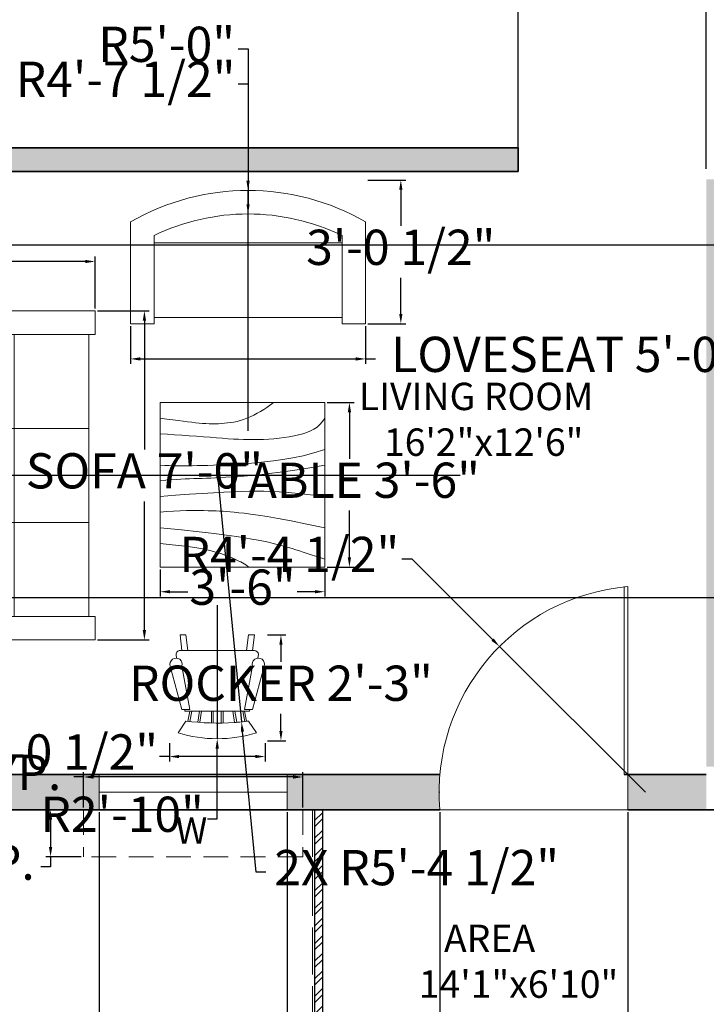
# Model space of a CAD drawing. Units: inches. Extents: x 9689 to 10369, y 10965 to 11626.
# Tile 3 of 11: x 9830 to 10005, y 11108 to 11359. Entities that reach past the tile are written whole.
import ezdxf

# ---------------------------------------------------------------- set-up
doc = ezdxf.new("R2010")
doc.units = ezdxf.units.IN
doc.linetypes.add('ACAD_ISO02W100', pattern=[15, 12, -3])
doc.linetypes.add('DASHED2', pattern=[9.525, 6.35, -3.175])
for name, color, linetype, lineweight in [('A-ANNO-DIMS', 2, 'Continuous', 18), ('A-ANNO-TEXT', 7, 'Continuous', 18), ('A-AREA-IDEN', 7, 'Continuous', 18), ('A-DOOR', 4, 'Continuous', 18), ('A-FLOR', 7, 'Continuous', 25), ('A-FLOR-PATT', 252, 'Continuous', 13), ('A-FURN', 8, 'Continuous', 18), ('A-GLAZ', 4, 'Continuous', 18), ('A-GLAZ-OVHD', 4, 'DASHED2', 13), ('A-WALL', 7, 'Continuous', 35), ('A-WALL-PATT', 252, 'Continuous', 13), ('C-PARK', 7, 'ACAD_ISO02W100', 18)]:
    doc.layers.add(name, color=color, linetype=linetype, lineweight=lineweight)
doc.styles.get("Standard").update_dxf_attribs({"font": 'arial.ttf'})
doc.dimstyles.new('ISO-25', dxfattribs={"dimtxt": 9, "dimasz": 2.5, "dimexe": 1.25, "dimexo": 0.625, "dimgap": 2, "dimtad": 0, "dimtih": 1, "dimtoh": 1, "dimdec": 1, "dimlunit": 4, "dimtxsty": 'Standard', "dimcen": 2.5, "dimadec": 0, "dimazin": 0, "dimtfac": 0.5, "dimtdec": 1, "dimtmove": 0, "dimatfit": 3, "dimfxl": 1, "dimarcsym": 0})

# ---------------------------------------------------------------- blocks, each defined once
blk = doc.blocks.new('Sofa - Roundback 7 ft.')
for p, q in [((-12.00002, -32.4421), (-12.00003, -6.5971)), ((11.99997, -32.4421), (11.99998, -6.5971)), ((-36.000027, -34), (-36.000027, -11.4696)), ((35.99998, -34), (35.99998, -11.4696)), ((-35.999844, -13.3819), (35.9998, -13.3819)), ((-36.000027, -32.4421), (35.99998, -32.4421))]:
    blk.add_line(p, q)
for points in [[(-36.000027, -34), (-42.000027, -34), (-42.000027, -8)], [(41.99998, -8), (41.99998, -34), (35.99998, -34)]]:
    blk.add_lwpolyline(points)
for centre, radius, start, end in [((0, -114.25), 114.25, 68.43141, 111.5686), ((-0.00001, -127.1968), 121.1968, 72.72033, 107.2797)]:
    blk.add_arc(centre, radius, start, end)
blk = doc.blocks.new('Sofa - Roundback Loveseat 5 ft.')
for p, q in [((0, -32.44198), (0, -5.99998)), ((-24, -33.99998), (-24, -11.46958)), ((24.00004, -33.99998), (24.00004, -11.46958)), ((-23.9998, -13.38178), (23.99986, -13.38178)), ((-24, -32.44198), (24.00004, -32.44198))]:
    blk.add_line(p, q)
for points in [[(-24, -33.99998), (-30, -33.99998), (-30, -7.99998)], [(30.00004, -7.99998), (30.00004, -33.99998), (24.00004, -33.99998)]]:
    blk.add_lwpolyline(points)
for centre, radius, start, end in [((0, -60.24998), 60.24998, 60.13715, 119.8628), ((0, -61.38438), 55.38444, 64.32083, 115.6792)]:
    blk.add_arc(centre, radius, start, end)
blk = doc.blocks.new('Chair - Rocking')
for p, q in [((-8, -4.5), (-10, -1.5)), ((8, -4.5), (10, -1.5)), ((-7.5, -4.5), (-7, -7)), ((-6.5, -7), (-7.02225, -4.43)), ((-4.5, -7), (-4.96674, -4.19951)), ((-4, -7), (-4.40532, -4.16272)), ((-1.5, -4.05012), (-1.5, -7)), ((-1, -7), (-1, -4.05012)), ((1, -7), (1, -4.04655)), ((1.5, -4.05012), (1.5, -7)), ((4, -7), (4.40187, -4.18694)), ((4.5, -7), (4.96761, -4.19437)), ((6.5, -7), (7, -4.4057)), ((7.5, -4.5), (7, -7)), ((-9, -7.5), (-12, -18.49999)), ((-7, -7.5), (-9, -7.5)), ((-9, -18.49999), (-7, -7.5)), ((-8.23428, -6.99939), (-8.3093, -7.47958)), ((-8.23041, -7), (8.23915, -7)), ((7, -7.5), (9, -7.5)), ((9, -18.49999), (7, -7.5)), ((8.31071, -7.48854), (8.23449, -7.00073)), ((9, -7.5), (12, -18.49999)), ((-10.36644, -20.64523), (-10.5, -21.49999)), ((-9, -22.49999), (-9.5, -26.49999)), ((0, -22.49999), (-9.5, -22.49999)), ((-8, -26.49999), (-7.5, -22.49999)), ((0, -22.49999), (9.5, -22.49999)), ((8, -26.49999), (7.5, -22.49999)), ((9, -22.49999), (9.5, -26.49999)), ((10.5, -21.49999), (10.3575, -20.58798)), ((-9.5, -26.49999), (-8, -26.49999)), ((9.5, -26.49999), (8, -26.49999))]:
    blk.add_line(p, q)
for centre, radius, start, end in [((0, -34.08333), 34.08333, 72.93847, 107.0615), ((0, -68.25004), 64.25, 93.92211, 97.15267), ((0, -68.25004), 64.25, 82.84733, 93.92211), ((-10.5, -18.99999), 1.58114, 161.5651, 18.43495), ((10.5, -18.99999), 1.58114, 161.5651, 18.43495), ((-9.5, -21.49999), 1, 180, 270), ((9.5, -21.49999), 1, 270, 0)]:
    blk.add_arc(centre, radius, start, end)
blk = doc.blocks.new('Table - Square Woodgrain 42 x 42 in.')
blk.add_line((0, -42), (42, -42))
for points in [[(0, -4), (1.704, -4.2172), (3.2358, -4.4188), (4.615, -4.604), (5.8615, -4.7721), (6.9951, -4.9224), (8.0357, -5.0541), (9.0031, -5.1667), (9.9171, -5.2594), (10.7951, -5.3316), (11.6445, -5.3836), (12.4702, -5.4157), (13.277, -5.4283), (14.0698, -5.4217), (14.8535, -5.3964), (15.6331, -5.3526), (16.4133, -5.2908), (17.1986, -5.2103), (17.9913, -5.1062), (18.793, -4.9727), (19.6056, -4.8038), (20.4307, -4.5937), (21.2701, -4.3365), (22.1256, -4.0262), (22.9989, -3.6571), (23.888, -3.2272), (24.7756, -2.7516), (25.6408, -2.2491), (26.4624, -1.7387), (27.2195, -1.2395), (27.891, -0.7703), (28.456, -0.3501), (28.8934, 0.002)], [(0, -42), (0, 0), (42, 0), (42, -42)], [(0, -8), (1.8203, -8.1001), (3.6741, -8.2149), (5.5411, -8.3408), (7.4011, -8.4741), (9.2339, -8.6112), (11.0193, -8.7484), (12.7371, -8.8821), (14.3671, -9.0086), (15.8954, -9.1246), (17.3337, -9.2278), (18.6997, -9.3159), (20.0116, -9.387), (21.2871, -9.4389), (22.5442, -9.4696), (23.8008, -9.477), (25.0749, -9.459), (26.3791, -9.4137), (27.7049, -9.3403), (29.0383, -9.2382), (30.3655, -9.1068), (31.6728, -8.9455), (32.9461, -8.7535), (34.1717, -8.5304), (35.3358, -8.2756), (36.4268, -7.9863), (37.443, -7.6521), (38.3849, -7.2603), (39.253, -6.7986), (40.048, -6.2542), (40.7705, -5.6147), (41.421, -4.8674), (42, -4)], [(42, -12), (39.1784, -12.8621), (36.4519, -13.5654), (33.8246, -14.1294), (31.3004, -14.5731), (28.8832, -14.9161), (26.577, -15.1775), (24.3858, -15.3768), (22.3136, -15.5332), (20.3622, -15.6632), (18.5254, -15.7718), (16.7947, -15.8612), (15.1618, -15.9338), (13.6183, -15.9916), (12.1558, -16.0369), (10.7659, -16.0718), (9.4403, -16.0987), (8.1703, -16.1191), (6.9461, -16.1325), (5.7577, -16.1377), (4.595, -16.1335), (3.4479, -16.1188), (2.3064, -16.0924), (1.1604, -16.0532), (0, -16)], [(42, -16), (37.6529, -16.7365), (33.8802, -17.329), (30.6179, -17.7961), (27.8015, -18.1561), (25.3668, -18.4275), (23.2497, -18.6288), (21.3859, -18.7785), (19.7111, -18.8949), (18.1693, -18.9939), (16.7375, -19.0795), (15.401, -19.1534), (14.1449, -19.217), (12.9544, -19.2717), (11.8148, -19.3191), (10.7113, -19.3606), (9.6291, -19.3976), (8.5534, -19.4323), (7.47, -19.4689), (6.3643, -19.5122), (5.222, -19.5672), (4.0288, -19.6386), (2.7703, -19.7313), (1.4321, -19.8501), (0, -20)], [(0, -24), (3.9243, -23.6805), (7.4766, -23.4138), (10.6891, -23.1954), (13.5943, -23.0205), (16.2247, -22.8847), (18.6125, -22.7832), (20.7903, -22.7116), (22.7903, -22.6651), (24.6563, -22.642), (26.4764, -22.6507), (28.35, -22.7024), (30.3766, -22.8084), (32.6555, -22.98), (35.2861, -23.2283), (38.3678, -23.5645), (42, -24)], [(42, -32), (37.392, -31.017), (33.4585, -30.2231), (30.1291, -29.5949), (27.3334, -29.109), (25.0009, -28.742), (23.0612, -28.4707), (21.4439, -28.2716), (20.0786, -28.1215), (18.8998, -28.0002), (17.8609, -27.9014), (16.9206, -27.8219), (16.0371, -27.7588), (15.1691, -27.709), (14.2748, -27.6693), (13.3128, -27.6368), (12.2415, -27.6083), (11.0295, -27.5824), (9.6867, -27.5643), (8.233, -27.5608), (6.6884, -27.5787), (5.0728, -27.6248), (3.4062, -27.7058), (1.7086, -27.8286), (0, -28)], [(0, -32), (5.4026, -32.5358), (9.9494, -33.019), (13.7424, -33.4553), (16.8834, -33.8505), (19.4743, -34.2106), (21.6171, -34.5413), (23.4136, -34.8486), (24.9657, -35.1382), (26.3614, -35.4156), (27.6332, -35.6841), (28.7995, -35.9467), (29.8788, -36.2064), (30.8897, -36.4661), (31.8507, -36.7288), (32.7802, -36.9973), (33.6968, -37.2747), (34.6175, -37.5635), (35.5531, -37.8651), (36.5128, -38.1805), (37.506, -38.5108), (38.5421, -38.8568), (39.6302, -39.2197), (40.7797, -39.6004), (42, -40)], [(0, -36), (3.0098, -36.2857), (5.5354, -36.5643), (7.6368, -36.8359), (9.374, -37.1009), (10.807, -37.3597), (11.9957, -37.6126), (13.0002, -37.8599), (13.8804, -38.102), (14.6874, -38.3393), (15.4365, -38.5729), (16.1338, -38.8041), (16.7858, -39.0341), (17.3987, -39.264), (17.9787, -39.4952), (18.5322, -39.7288), (19.0655, -39.9662), (19.5832, -40.2081), (20.0842, -40.4544), (20.5657, -40.7046), (21.0249, -40.9581), (21.459, -41.2144), (21.8653, -41.4731), (22.2409, -41.7335), (22.5831, -41.9951)]]:
    blk.add_lwpolyline(points)
blk = doc.blocks.new('WINDOW-HOOD-56')
for p, q in [((0, 0), (0, 12)), ((0, 12), (56, 12)), ((56, 0), (56, 12))]:
    blk.add_line(p, q)
blk = doc.blocks.new('WINDOW-48')
for p, q in [((0, 0), (0, 9)), ((48, 0), (48, 9)), ((0, 4.5), (48, 4.5))]:
    blk.add_line(p, q)
blk = doc.blocks.new('*D38')
at = {"layer": 'A-ANNO-DIMS', "color": 0, "lineweight": -2, "transparency": 16777216}
for p, q in [((9846.06, 11166.03), (9843.56, 11166.03)), ((9846.06, 11158.26), (9846.06, 11167.28)), ((9899.56, 11166.03), (9848.56, 11166.03)), ((9902.06, 11158.26), (9902.06, 11167.28))]:
    blk.add_line(p, q, dxfattribs=at)
at = {"layer": 'A-ANNO-DIMS', "color": 0, "transparency": 16777216}
for points in [[(9848.56, 11166.45), (9848.56, 11165.61), (9846.06, 11166.03)], [(9899.56, 11166.45), (9899.56, 11165.61), (9902.06, 11166.03)]]:
    blk.add_solid(points, dxfattribs=at)
at = {"layer": 'Defpoints', "color": 0, "transparency": 16777216}
for p in [(9846.06, 11166.03), (9846.06, 11157.63), (9902.06, 11157.63)]:
    blk.add_point(p, dxfattribs=at)
at = {"layer": 'A-ANNO-DIMS', "color": 0, "transparency": 16777216, "insert": (9793.76, 11166.03), "char_height": 9, "attachment_point": 5}
blk.add_mtext('HOOD 4\'-8" TYP.', dxfattribs=at)
blk = doc.blocks.new('*D39')
at = {"layer": 'A-ANNO-DIMS', "color": 0, "lineweight": -2, "transparency": 16777216}
for p, q in [((9845.43, 11157.63), (9836.41, 11157.63)), ((9837.66, 11155.13), (9837.66, 11148.13)), ((9845.43, 11145.63), (9836.41, 11145.63)), ((9837.66, 11145.63), (9837.66, 11143.13)), ((9837.66, 11143.13), (9835.16, 11143.13))]:
    blk.add_line(p, q, dxfattribs=at)
at = {"layer": 'A-ANNO-DIMS', "color": 0, "transparency": 16777216}
for points in [[(9837.24, 11155.13), (9838.07, 11155.13), (9837.66, 11157.63)], [(9837.24, 11148.13), (9838.07, 11148.13), (9837.66, 11145.63)]]:
    blk.add_solid(points, dxfattribs=at)
at = {"layer": 'Defpoints', "color": 0, "transparency": 16777216}
for p in [(9846.06, 11157.63), (9837.66, 11145.63), (9846.06, 11145.63)]:
    blk.add_point(p, dxfattribs=at)
at = {"layer": 'A-ANNO-DIMS', "color": 0, "transparency": 16777216, "insert": (9806.15, 11143.13), "char_height": 9, "attachment_point": 5}
blk.add_mtext('1\'-0" TYP.', dxfattribs=at)
blk = doc.blocks.new('*D54')
at = {"layer": 'A-ANNO-DIMS', "color": 0, "lineweight": -2, "transparency": 16777216}
for p, q in [((9849.64, 11285.02), (9862.86, 11285.02)), ((9861.61, 11282.52), (9861.61, 11249.67)), ((9861.61, 11203.52), (9861.61, 11236.36)), ((9849.64, 11201.02), (9862.86, 11201.02))]:
    blk.add_line(p, q, dxfattribs=at)
at = {"layer": 'A-ANNO-DIMS', "color": 0, "transparency": 16777216}
for points in [[(9861.19, 11282.52), (9862.03, 11282.52), (9861.61, 11285.02)], [(9861.19, 11203.52), (9862.03, 11203.52), (9861.61, 11201.02)]]:
    blk.add_solid(points, dxfattribs=at)
at = {"layer": 'Defpoints', "color": 0, "transparency": 16777216}
for p in [(9849.01, 11285.02), (9861.61, 11285.02), (9849.01, 11201.02)]:
    blk.add_point(p, dxfattribs=at)
at = {"layer": 'A-ANNO-DIMS', "color": 0, "transparency": 16777216, "insert": (9861.61, 11243.02), "char_height": 9, "attachment_point": 5}
blk.add_mtext('SOFA 7\'-0"', dxfattribs=at)
blk = doc.blocks.new('*D55')
at = {"layer": 'A-ANNO-DIMS', "color": 0, "lineweight": -2, "transparency": 16777216}
for p, q in [((9812.34, 11285.64), (9812.34, 11298.87)), ((9849.01, 11285.64), (9849.01, 11298.87)), ((9812.34, 11297.62), (9809.84, 11297.62)), ((9846.51, 11297.62), (9814.84, 11297.62))]:
    blk.add_line(p, q, dxfattribs=at)
at = {"layer": 'A-ANNO-DIMS', "color": 0, "transparency": 16777216}
for points in [[(9814.84, 11298.03), (9814.84, 11297.2), (9812.34, 11297.62)], [(9846.51, 11298.03), (9846.51, 11297.2), (9849.01, 11297.62)]]:
    blk.add_solid(points, dxfattribs=at)
at = {"layer": 'Defpoints', "color": 0, "transparency": 16777216}
for p in [(9812.34, 11297.62), (9812.34, 11285.02), (9849.01, 11285.02)]:
    blk.add_point(p, dxfattribs=at)
at = {"layer": 'A-ANNO-DIMS', "color": 0, "transparency": 16777216, "insert": (9785.4, 11297.62), "char_height": 9, "attachment_point": 5}
blk.add_mtext('3\'-0 1/2"', dxfattribs=at)
blk = doc.blocks.new('*D56')
at = {"layer": 'A-ANNO-DIMS', "color": 0, "lineweight": -2, "transparency": 16777216}
for p, q in [((9858.07, 11281.13), (9858.07, 11271.5)), ((9918.07, 11281.13), (9918.07, 11271.5)), ((9860.57, 11272.75), (9915.57, 11272.75)), ((9918.07, 11272.75), (9920.57, 11272.75))]:
    blk.add_line(p, q, dxfattribs=at)
at = {"layer": 'A-ANNO-DIMS', "color": 0, "transparency": 16777216}
for points in [[(9860.57, 11273.17), (9860.57, 11272.33), (9858.07, 11272.75)], [(9915.57, 11273.17), (9915.57, 11272.33), (9918.07, 11272.75)]]:
    blk.add_solid(points, dxfattribs=at)
at = {"layer": 'Defpoints', "color": 0, "transparency": 16777216}
for p in [(9858.07, 11281.75), (9918.07, 11281.75), (9918.07, 11272.75)]:
    blk.add_point(p, dxfattribs=at)
at = {"layer": 'A-ANNO-DIMS', "color": 0, "transparency": 16777216, "insert": (9969.27, 11272.75), "char_height": 9, "attachment_point": 5}
blk.add_mtext('LOVESEAT 5\'-0"', dxfattribs=at)
blk = doc.blocks.new('*D57')
at = {"layer": 'A-ANNO-DIMS', "color": 0, "lineweight": -2, "transparency": 16777216}
for p, q in [((9918.69, 11318.42), (9928.32, 11318.42)), ((9927.07, 11315.92), (9927.07, 11306.74)), ((9927.07, 11284.25), (9927.07, 11293.43)), ((9918.69, 11281.75), (9928.32, 11281.75))]:
    blk.add_line(p, q, dxfattribs=at)
at = {"layer": 'A-ANNO-DIMS', "color": 0, "transparency": 16777216}
for points in [[(9926.65, 11315.92), (9927.49, 11315.92), (9927.07, 11318.42)], [(9926.65, 11284.25), (9927.49, 11284.25), (9927.07, 11281.75)]]:
    blk.add_solid(points, dxfattribs=at)
at = {"layer": 'Defpoints', "color": 0, "transparency": 16777216}
for p in [(9918.07, 11318.42), (9927.07, 11318.42), (9918.07, 11281.75)]:
    blk.add_point(p, dxfattribs=at)
at = {"layer": 'A-ANNO-DIMS', "color": 0, "transparency": 16777216, "insert": (9927.07, 11300.08), "char_height": 9, "attachment_point": 5}
blk.add_mtext('3\'-0 1/2"', dxfattribs=at)
blk = doc.blocks.new('*D58')
at = {"layer": 'A-ANNO-DIMS', "color": 0, "lineweight": -2, "transparency": 16777216}
for p, q in [((9893.04, 11202.3), (9897.72, 11202.3)), ((9896.47, 11199.8), (9896.47, 11195.46)), ((9896.47, 11177.8), (9896.47, 11182.14)), ((9893.04, 11175.3), (9897.72, 11175.3))]:
    blk.add_line(p, q, dxfattribs=at)
at = {"layer": 'A-ANNO-DIMS', "color": 0, "transparency": 16777216}
for points in [[(9896.05, 11199.8), (9896.88, 11199.8), (9896.47, 11202.3)], [(9896.05, 11177.8), (9896.88, 11177.8), (9896.47, 11175.3)]]:
    blk.add_solid(points, dxfattribs=at)
at = {"layer": 'Defpoints', "color": 0, "transparency": 16777216}
for p in [(9892.42, 11202.3), (9892.42, 11175.3), (9896.47, 11175.3)]:
    blk.add_point(p, dxfattribs=at)
at = {"layer": 'A-ANNO-DIMS', "color": 0, "transparency": 16777216, "insert": (9896.47, 11188.8), "char_height": 9, "attachment_point": 5}
blk.add_mtext('ROCKER 2\'-3"', dxfattribs=at)
blk = doc.blocks.new('*D59')
at = {"layer": 'A-ANNO-DIMS', "color": 0, "lineweight": -2, "transparency": 16777216}
for p, q in [((9867.98, 11174.67), (9867.98, 11170)), ((9892.42, 11174.67), (9892.42, 11170)), ((9867.98, 11171.25), (9865.48, 11171.25)), ((9889.92, 11171.25), (9870.48, 11171.25))]:
    blk.add_line(p, q, dxfattribs=at)
at = {"layer": 'A-ANNO-DIMS', "color": 0, "transparency": 16777216}
for points in [[(9870.48, 11171.67), (9870.48, 11170.83), (9867.98, 11171.25)], [(9889.92, 11171.67), (9889.92, 11170.83), (9892.42, 11171.25)]]:
    blk.add_solid(points, dxfattribs=at)
at = {"layer": 'Defpoints', "color": 0, "transparency": 16777216}
for p in [(9867.98, 11175.3), (9892.42, 11175.3), (9867.98, 11171.25)]:
    blk.add_point(p, dxfattribs=at)
at = {"layer": 'A-ANNO-DIMS', "color": 0, "transparency": 16777216, "insert": (9840.96, 11171.25), "char_height": 9, "attachment_point": 5}
blk.add_mtext('2\'-0 1/2"', dxfattribs=at)
blk = doc.blocks.new('*D60')
at = {"layer": 'A-ANNO-DIMS', "color": 0, "lineweight": -2, "transparency": 16777216}
for p, q in [((9908.27, 11261.62), (9915.2, 11261.62)), ((9913.95, 11259.12), (9913.95, 11247.22)), ((9913.95, 11222.12), (9913.95, 11234.03)), ((9908.27, 11219.62), (9915.2, 11219.62))]:
    blk.add_line(p, q, dxfattribs=at)
at = {"layer": 'A-ANNO-DIMS', "color": 0, "transparency": 16777216}
for points in [[(9913.53, 11259.12), (9914.37, 11259.12), (9913.95, 11261.62)], [(9913.53, 11222.12), (9914.37, 11222.12), (9913.95, 11219.62)]]:
    blk.add_solid(points, dxfattribs=at)
at = {"layer": 'Defpoints', "color": 0, "transparency": 16777216}
for p in [(9907.65, 11261.62), (9913.95, 11261.62), (9907.65, 11219.62)]:
    blk.add_point(p, dxfattribs=at)
at = {"layer": 'A-ANNO-DIMS', "color": 0, "transparency": 16777216, "insert": (9913.95, 11240.62), "char_height": 9, "attachment_point": 5}
blk.add_mtext('TABLE 3\'-6"', dxfattribs=at)
blk = doc.blocks.new('*D61')
at = {"layer": 'A-ANNO-DIMS', "color": 0, "lineweight": -2, "transparency": 16777216}
for p, q in [((9865.65, 11219), (9865.65, 11212.07)), ((9907.65, 11219), (9907.65, 11212.07)), ((9868.15, 11213.32), (9872.69, 11213.32)), ((9905.15, 11213.32), (9900.61, 11213.32))]:
    blk.add_line(p, q, dxfattribs=at)
at = {"layer": 'A-ANNO-DIMS', "color": 0, "transparency": 16777216}
for points in [[(9868.15, 11213.74), (9868.15, 11212.91), (9865.65, 11213.32)], [(9905.15, 11213.74), (9905.15, 11212.91), (9907.65, 11213.32)]]:
    blk.add_solid(points, dxfattribs=at)
at = {"layer": 'Defpoints', "color": 0, "transparency": 16777216}
for p in [(9865.65, 11219.62), (9907.65, 11219.62), (9907.65, 11213.32)]:
    blk.add_point(p, dxfattribs=at)
at = {"layer": 'A-ANNO-DIMS', "color": 0, "transparency": 16777216, "insert": (9886.65, 11213.32), "char_height": 9, "attachment_point": 5}
blk.add_mtext('3\'-6"', dxfattribs=at)
blk = doc.blocks.new('*D67')
at = {"layer": 'A-ANNO-DIMS', "color": 0, "lineweight": -2, "transparency": 16777216}
for p, q in [((9802.06, 11157.01), (9802.06, 10977.48)), ((9905.06, 11157.01), (9905.06, 10977.48)), ((9804.56, 10978.73), (9839.59, 10978.73)), ((9902.56, 10978.73), (9867.53, 10978.73))]:
    blk.add_line(p, q, dxfattribs=at)
at = {"layer": 'A-ANNO-DIMS', "color": 0, "transparency": 16777216}
for points in [[(9804.56, 10979.15), (9804.56, 10978.31), (9802.06, 10978.73)], [(9902.56, 10979.15), (9902.56, 10978.31), (9905.06, 10978.73)]]:
    blk.add_solid(points, dxfattribs=at)
at = {"layer": 'Defpoints', "color": 0, "transparency": 16777216}
for p in [(9802.06, 11157.63), (9905.06, 11157.63), (9905.06, 10978.73)]:
    blk.add_point(p, dxfattribs=at)
at = {"layer": 'A-ANNO-DIMS', "color": 0, "transparency": 16777216, "insert": (9853.56, 10978.73), "char_height": 9, "attachment_point": 5}
blk.add_mtext('8\'-7"', dxfattribs=at)
blk = doc.blocks.new('*D73')
at = {"layer": 'A-ANNO-DIMS', "color": 0, "lineweight": -2, "transparency": 16777216}
for p, q in [((10010.43, 11301.79), (9758.91, 11301.79)), ((9760.16, 11299.29), (9760.16, 11263.38)), ((9760.16, 11214.29), (9760.16, 11250.19)), ((10010.43, 11211.79), (9758.91, 11211.79))]:
    blk.add_line(p, q, dxfattribs=at)
at = {"layer": 'A-ANNO-DIMS', "color": 0, "transparency": 16777216}
for points in [[(9759.74, 11299.29), (9760.57, 11299.29), (9760.16, 11301.79)], [(9759.74, 11214.29), (9760.57, 11214.29), (9760.16, 11211.79)]]:
    blk.add_solid(points, dxfattribs=at)
at = {"layer": 'Defpoints', "color": 0, "transparency": 16777216}
for p in [(9760.16, 11301.79), (10011.06, 11301.79), (10011.06, 11211.79)]:
    blk.add_point(p, dxfattribs=at)
at = {"layer": 'A-ANNO-DIMS', "color": 0, "transparency": 16777216, "insert": (9760.16, 11256.79), "char_height": 9, "attachment_point": 5}
blk.add_mtext('7\'-6"', dxfattribs=at)
blk = doc.blocks.new('*D85')
at = {"layer": 'A-ANNO-DIMS', "color": 0, "lineweight": -2, "transparency": 16777216}
for p, q in [((9937.06, 11157.01), (9937.06, 10977.48)), ((9985.06, 11157.01), (9985.06, 10977.48)), ((9939.56, 10978.73), (9946.91, 10978.73)), ((9982.56, 10978.73), (9975.2, 10978.73))]:
    blk.add_line(p, q, dxfattribs=at)
at = {"layer": 'A-ANNO-DIMS', "color": 0, "transparency": 16777216}
for points in [[(9939.56, 10979.15), (9939.56, 10978.31), (9937.06, 10978.73)], [(9982.56, 10979.15), (9982.56, 10978.31), (9985.06, 10978.73)]]:
    blk.add_solid(points, dxfattribs=at)
at = {"layer": 'Defpoints', "color": 0, "transparency": 16777216}
for p in [(9937.06, 11157.63), (9985.06, 11157.63), (9985.06, 10978.73)]:
    blk.add_point(p, dxfattribs=at)
at = {"layer": 'A-ANNO-DIMS', "color": 0, "transparency": 16777216, "insert": (9961.06, 10978.73), "char_height": 9, "attachment_point": 5}
blk.add_mtext('4\'-0"', dxfattribs=at)
blk = doc.blocks.new('*D87')
at = {"layer": 'A-ANNO-DIMS', "color": 0, "lineweight": -2, "transparency": 16777216}
for p, q in [((9802.06, 11157.01), (9802.06, 10977.48)), ((9850.06, 11157.01), (9850.06, 10977.48)), ((9804.56, 10978.73), (9811.91, 10978.73)), ((9847.56, 10978.73), (9840.2, 10978.73))]:
    blk.add_line(p, q, dxfattribs=at)
at = {"layer": 'A-ANNO-DIMS', "color": 0, "transparency": 16777216}
for points in [[(9804.56, 10979.15), (9804.56, 10978.31), (9802.06, 10978.73)], [(9847.56, 10979.15), (9847.56, 10978.31), (9850.06, 10978.73)]]:
    blk.add_solid(points, dxfattribs=at)
at = {"layer": 'Defpoints', "color": 0, "transparency": 16777216}
for p in [(9802.06, 11157.63), (9850.06, 11157.63), (9850.06, 10978.73)]:
    blk.add_point(p, dxfattribs=at)
at = {"layer": 'A-ANNO-DIMS', "color": 0, "transparency": 16777216, "insert": (9826.06, 10978.73), "char_height": 9, "attachment_point": 5}
blk.add_mtext('4\'-0"', dxfattribs=at)
blk = doc.blocks.new('*D88')
at = {"layer": 'A-ANNO-DIMS', "color": 0, "lineweight": -2, "transparency": 16777216}
for p, q in [((9898.06, 11157.01), (9898.06, 10977.48)), ((9937.06, 11157.01), (9937.06, 10977.48)), ((9900.56, 10978.73), (9903.6, 10978.73)), ((9934.56, 10978.73), (9931.52, 10978.73))]:
    blk.add_line(p, q, dxfattribs=at)
at = {"layer": 'A-ANNO-DIMS', "color": 0, "transparency": 16777216}
for points in [[(9900.56, 10979.15), (9900.56, 10978.31), (9898.06, 10978.73)], [(9934.56, 10979.15), (9934.56, 10978.31), (9937.06, 10978.73)]]:
    blk.add_solid(points, dxfattribs=at)
at = {"layer": 'Defpoints', "color": 0, "transparency": 16777216}
for p in [(9898.06, 11157.63), (9937.06, 11157.63), (9937.06, 10978.73)]:
    blk.add_point(p, dxfattribs=at)
at = {"layer": 'A-ANNO-DIMS', "color": 0, "transparency": 16777216, "insert": (9917.56, 10978.73), "char_height": 9, "attachment_point": 5}
blk.add_mtext('3\'-3"', dxfattribs=at)
blk = doc.blocks.new('*D97')
at = {"layer": 'A-ANNO-DIMS', "color": 0, "lineweight": -2, "transparency": 16777216}
for p, q in [((9957.06, 11321.26), (9957.06, 11613.7)), ((9959.56, 11612.45), (9966.91, 11612.45)), ((10002.56, 11612.45), (9995.2, 11612.45)), ((10005.06, 11321.26), (10005.06, 11613.7))]:
    blk.add_line(p, q, dxfattribs=at)
at = {"layer": 'A-ANNO-DIMS', "color": 0, "transparency": 16777216}
for points in [[(9959.56, 11612.87), (9959.56, 11612.04), (9957.06, 11612.45)], [(10002.56, 11612.87), (10002.56, 11612.04), (10005.06, 11612.45)]]:
    blk.add_solid(points, dxfattribs=at)
at = {"layer": 'Defpoints', "color": 0, "transparency": 16777216}
for p in [(10005.06, 11612.45), (9957.06, 11320.63), (10005.06, 11320.63)]:
    blk.add_point(p, dxfattribs=at)
at = {"layer": 'A-ANNO-DIMS', "color": 0, "transparency": 16777216, "insert": (9981.06, 11612.45), "char_height": 9, "attachment_point": 5}
blk.add_mtext('4\'-0"', dxfattribs=at)
blk = doc.blocks.new('*D99')
at = {"layer": 'A-ANNO-DIMS', "color": 0, "lineweight": -2, "transparency": 16777216}
for p, q in [((9922.43, 11374.63), (9758.91, 11374.63)), ((9760.16, 11372.13), (9760.16, 11357.23)), ((9760.16, 11329.13), (9760.16, 11344.03)), ((9801.43, 11326.63), (9758.91, 11326.63))]:
    blk.add_line(p, q, dxfattribs=at)
at = {"layer": 'A-ANNO-DIMS', "color": 0, "transparency": 16777216}
for points in [[(9759.74, 11372.13), (9760.57, 11372.13), (9760.16, 11374.63)], [(9759.74, 11329.13), (9760.57, 11329.13), (9760.16, 11326.63)]]:
    blk.add_solid(points, dxfattribs=at)
at = {"layer": 'Defpoints', "color": 0, "transparency": 16777216}
for p in [(9923.06, 11374.63), (9760.16, 11326.63), (9802.06, 11326.63)]:
    blk.add_point(p, dxfattribs=at)
at = {"layer": 'A-ANNO-DIMS', "color": 0, "transparency": 16777216, "insert": (9760.16, 11350.63), "char_height": 9, "attachment_point": 5}
blk.add_mtext('4\'-0"', dxfattribs=at)
blk = doc.blocks.new('*D121')
at = {"layer": 'A-ANNO-DIMS', "color": 0, "lineweight": -2, "transparency": 16777216}
for p, q in [((9927.37, 11221.68), (9929.87, 11221.68)), ((9929.87, 11221.68), (9950.49, 11201.11)), ((9989.56, 11162.13), (9952.26, 11199.35))]:
    blk.add_line(p, q, dxfattribs=at)
at = {"layer": 'A-ANNO-DIMS', "color": 0, "transparency": 16777216}
blk.add_solid([(9950.78, 11201.41), (9950.19, 11200.82), (9952.26, 11199.35)], dxfattribs=at)
at = {"layer": 'Defpoints', "color": 0, "transparency": 16777216}
for p in [(9952.26, 11199.35), (9989.56, 11162.13)]:
    blk.add_point(p, dxfattribs=at)
at = {"layer": 'A-ANNO-DIMS', "color": 0, "transparency": 16777216, "insert": (9898.62, 11221.68), "char_height": 9, "attachment_point": 5}
blk.add_mtext('R4\'-4 1/2"', dxfattribs=at)
blk = doc.blocks.new('*D124')
at = {"layer": 'A-ANNO-DIMS', "color": 0, "lineweight": -2, "transparency": 16777216}
for p, q in [((9746.46, 11243.02), (9812.51, 11243.02)), ((9929.26, 11243.02), (9815.01, 11243.02))]:
    blk.add_line(p, q, dxfattribs=at)
at = {"layer": 'A-ANNO-DIMS', "color": 0, "transparency": 16777216}
blk.add_solid([(9812.51, 11243.43), (9812.51, 11242.6), (9815.01, 11243.02)], dxfattribs=at)
at = {"layer": 'Defpoints', "color": 0, "transparency": 16777216}
for p in [(9815.01, 11243.02), (9929.26, 11243.02)]:
    blk.add_point(p, dxfattribs=at)
at = {"layer": 'A-ANNO-DIMS', "color": 0, "transparency": 16777216, "insert": (9717.71, 11243.02), "char_height": 9, "attachment_point": 5}
blk.add_mtext('R9\'-6 1/2"', dxfattribs=at)
blk = doc.blocks.new('*D125')
at = {"layer": 'A-ANNO-DIMS', "color": 0, "lineweight": -2, "transparency": 16777216}
for p, q in [((9748.29, 11243.02), (9818.51, 11243.02)), ((9942.21, 11243.02), (9821.01, 11243.02))]:
    blk.add_line(p, q, dxfattribs=at)
at = {"layer": 'A-ANNO-DIMS', "color": 0, "transparency": 16777216}
blk.add_solid([(9818.51, 11243.43), (9818.51, 11242.6), (9821.01, 11243.02)], dxfattribs=at)
at = {"layer": 'Defpoints', "color": 0, "transparency": 16777216}
for p in [(9821.01, 11243.02), (9942.21, 11243.02)]:
    blk.add_point(p, dxfattribs=at)
at = {"layer": 'A-ANNO-DIMS', "color": 0, "transparency": 16777216, "insert": (9726.53, 11243.02), "char_height": 9, "attachment_point": 5}
blk.add_mtext('R10\'-1"', dxfattribs=at)
blk = doc.blocks.new('*D126')
at = {"layer": 'A-ANNO-DIMS', "color": 0, "lineweight": -2, "transparency": 16777216}
for p, q in [((9885.57, 11351.9), (9888.07, 11351.9)), ((9888.07, 11351.9), (9888.07, 11318.25)), ((9888.07, 11255.5), (9888.07, 11315.75))]:
    blk.add_line(p, q, dxfattribs=at)
at = {"layer": 'A-ANNO-DIMS', "color": 0, "transparency": 16777216}
blk.add_solid([(9888.49, 11318.25), (9887.65, 11318.25), (9888.07, 11315.75)], dxfattribs=at)
at = {"layer": 'Defpoints', "color": 0, "transparency": 16777216}
for p in [(9888.07, 11315.75), (9888.07, 11255.5)]:
    blk.add_point(p, dxfattribs=at)
at = {"layer": 'A-ANNO-DIMS', "color": 0, "transparency": 16777216, "insert": (9867.3, 11351.9), "char_height": 9, "attachment_point": 5}
blk.add_mtext('R5\'-0"', dxfattribs=at)
blk = doc.blocks.new('*D127')
at = {"layer": 'A-ANNO-DIMS', "color": 0, "lineweight": -2, "transparency": 16777216}
for p, q in [((9885.57, 11342.98), (9888.07, 11342.98)), ((9888.07, 11342.98), (9888.07, 11312.25)), ((9888.07, 11254.37), (9888.07, 11309.75))]:
    blk.add_line(p, q, dxfattribs=at)
at = {"layer": 'A-ANNO-DIMS', "color": 0, "transparency": 16777216}
blk.add_solid([(9888.49, 11312.25), (9887.65, 11312.25), (9888.07, 11309.75)], dxfattribs=at)
at = {"layer": 'Defpoints', "color": 0, "transparency": 16777216}
for p in [(9888.07, 11309.75), (9888.07, 11254.37)]:
    blk.add_point(p, dxfattribs=at)
at = {"layer": 'A-ANNO-DIMS', "color": 0, "transparency": 16777216, "insert": (9856.81, 11342.98), "char_height": 9, "attachment_point": 5}
blk.add_mtext('R4\'-7 1/2"', dxfattribs=at)
blk = doc.blocks.new('*D128')
at = {"layer": 'A-ANNO-DIMS', "color": 0, "lineweight": -2, "transparency": 16777216}
for p, q in [((9880.2, 11244.05), (9886.4, 11180.1)), ((9890.12, 11141.73), (9886.64, 11177.61)), ((9892.62, 11141.73), (9890.12, 11141.73))]:
    blk.add_line(p, q, dxfattribs=at)
at = {"layer": 'A-ANNO-DIMS', "color": 0, "transparency": 16777216}
blk.add_solid([(9887.06, 11177.65), (9886.23, 11177.57), (9886.4, 11180.1)], dxfattribs=at)
at = {"layer": 'Defpoints', "color": 0, "transparency": 16777216}
for p in [(9880.2, 11244.05), (9886.4, 11180.1)]:
    blk.add_point(p, dxfattribs=at)
at = {"layer": 'A-ANNO-DIMS', "color": 0, "transparency": 16777216, "insert": (9931.12, 11141.73), "char_height": 9, "attachment_point": 5}
blk.add_mtext('2X R5\'-4 1/2"', dxfattribs=at)
blk = doc.blocks.new('*D129')
at = {"layer": 'A-ANNO-DIMS', "color": 0, "lineweight": -2, "transparency": 16777216}
for p, q in [((9880.2, 11209.88), (9880.2, 11175.8)), ((9880.2, 11155.35), (9880.2, 11173.3)), ((9877.7, 11155.35), (9880.2, 11155.35))]:
    blk.add_line(p, q, dxfattribs=at)
at = {"layer": 'A-ANNO-DIMS', "color": 0, "transparency": 16777216}
blk.add_solid([(9879.78, 11173.3), (9880.62, 11173.3), (9880.2, 11175.8)], dxfattribs=at)
at = {"layer": 'Defpoints', "color": 0, "transparency": 16777216}
for p in [(9880.2, 11209.88), (9880.2, 11175.8)]:
    blk.add_point(p, dxfattribs=at)
at = {"layer": 'A-ANNO-DIMS', "color": 0, "transparency": 16777216, "insert": (9855.93, 11155.35), "char_height": 9, "attachment_point": 5}
blk.add_mtext('R2\'-10"', dxfattribs=at)

msp = doc.modelspace()

# ---------------------------------------------------------------- hatches: boundary and pattern name
at = {"layer": 'A-FLOR-PATT'}
h = msp.add_hatch(dxfattribs=at)
h.set_pattern_fill('STEEL', color=256)
h.set_pattern_definition([(45, (0, 0), (-2.245064, 2.245064), []), (45, (0, 1.5875), (-2.245064, 2.245064), [])])
h.paths.add_polyline_path([(10074.06, 11157.63), (10072.06, 11157.63), (10072.06, 11077.63), (9985.06, 11077.63), (9985.06, 11075.63), (10074.06, 11075.63)])
h.paths.add_polyline_path([(9907.06, 11157.63), (9905.06, 11157.63), (9905.06, 11075.63), (9937.06, 11075.63), (9937.06, 11077.63), (9907.06, 11077.63)])
at = {"layer": 'A-WALL-PATT'}
h = msp.add_hatch(dxfattribs=at)
h.set_pattern_fill('ANSI33', color=256)
h.paths.add_polyline_path([(9843.06, 11538.63), (9811.06, 11538.63), (9811.06, 11529.63), (9843.06, 11529.63)])
h.paths.add_polyline_path([(9923.06, 11538.63), (9891.06, 11538.63), (9891.06, 11529.63), (9923.06, 11529.63)])
h.paths.add_polyline_path([(9929.06, 11527.63), (9923.06, 11527.63), (9923.06, 11380.63), (9929.06, 11380.63)])
h.paths.add_polyline_path([(9939.06, 11538.63), (9929.06, 11538.63), (9929.06, 11529.63), (9939.06, 11529.63, -0.071068)])
h.paths.add_polyline_path([(10035.06, 11538.63), (10013.06, 11538.63), (10013.06, 11529.63), (10022.06, 11529.63), (10022.06, 11507.38), (10022.06, 11502.38), (10022.06, 11482.38), (10022.06, 11478.38), (10022.06, 11456.13, -0.038405), (10026.06, 11456.13), (10026.06, 11502.38), (10026.06, 11529.63), (10035.06, 11529.63)])
h.paths.add_polyline_path([(10068.06, 11538.63), (10059.06, 11538.63), (10059.06, 11529.63), (10068.06, 11529.63)])
h.paths.add_polyline_path([(10074.06, 11527.63), (10068.06, 11527.63), (10068.06, 11431.13), (10026.06, 11431.13), (10022.06, 11431.13), (9980.06, 11431.13), (9976.06, 11431.13), (9976.06, 11425.13), (10068.06, 11425.13), (10068.06, 11380.63), (10074.06, 11380.63)])
h.paths.add_polyline_path([(10124.56, 11538.63), (10074.06, 11538.63), (10074.06, 11529.63), (10124.56, 11529.63)])
h.paths.add_polyline_path([(9980.06, 11507.38), (9980.06, 11529.63), (9989.06, 11529.63), (9989.06, 11538.63), (9976.06, 11538.63), (9976.06, 11529.63), (9976.06, 11503.38), (9976.06, 11483.38), (9976.06, 11478.38), (9980.06, 11478.38), (9997.06, 11478.38, -0.038405), (9997.06, 11482.38), (9980.06, 11482.38)])
h.paths.add_polyline_path([(10235.06, 11538.63), (10184.56, 11538.63), (10184.56, 11529.63), (10235.06, 11529.63)])
h.paths.add_polyline_path([(10244.06, 11527.63), (10235.06, 11527.63), (10235.06, 11485.13), (10244.06, 11485.13)])
h.paths.add_polyline_path([(10244.06, 11425.13), (10235.06, 11425.13), (10235.06, 11380.63), (10244.06, 11380.63)])
h.paths.add_polyline_path([(10233.06, 11380.63), (10120.06, 11380.63, -0.038405), (10120.06, 11374.63), (10133.04, 11374.63), (10133.04, 11326.63), (10120.06, 11326.63, -0.038405), (10120.06, 11320.63), (10149.19, 11320.63), (10149.19, 11326.63), (10136.04, 11326.63), (10136.04, 11374.63), (10233.06, 11374.63)])
h.paths.add_polyline_path([(10084.06, 11380.63), (10076.06, 11380.63), (10076.06, 11374.63), (10084.06, 11374.63)])
h.paths.add_polyline_path([(10244.06, 11374.63), (10235.06, 11374.63), (10235.06, 11362.63), (10244.06, 11362.63)])
h.paths.add_polyline_path([(10244.06, 11338.63), (10235.06, 11338.63), (10235.06, 11326.63), (10244.06, 11326.63)])
h.paths.add_polyline_path([(10233.06, 11326.63), (10173.19, 11326.63, -0.055385), (10173.19, 11320.63), (10233.06, 11320.63)], flags=0)
h.paths.add_polyline_path([(10244.06, 11320.63), (10235.06, 11320.63), (10235.06, 11273.63), (10244.06, 11273.63)])
h = msp.add_hatch(dxfattribs=at)
h.set_pattern_fill('ANSI36', color=256)
h.paths.add_polyline_path([(10233.06, 11326.63), (10173.19, 11326.63, -0.055385), (10173.19, 11320.63), (10233.06, 11320.63)])
h.paths.add_polyline_path([(10244.06, 11213.63), (10235.06, 11213.63), (10235.06, 11166.63), (10244.06, 11166.63)])
h.paths.add_polyline_path([(10233.06, 11166.63), (10184.56, 11166.63), (10184.56, 11157.63), (10233.06, 11157.63)])
h.paths.add_polyline_path([(10124.56, 11166.63), (10074.06, 11166.63), (10074.06, 11157.63), (10124.56, 11157.63)])
h.paths.add_polyline_path([(10074.06, 11318.63), (10068.06, 11318.63), (10068.06, 11168.63), (10074.06, 11168.63)])
h.paths.add_polyline_path([(10068.06, 11166.63), (10011.06, 11166.63), (10011.06, 11157.63), (10068.06, 11157.63)])
h.paths.add_polyline_path([(10011.06, 11318.63), (10005.06, 11318.63), (10005.06, 11168.63), (10011.06, 11168.63)])
h.paths.add_polyline_path([(10005.06, 11166.63), (9985.06, 11166.63), (9985.06, 11157.63), (10005.06, 11157.63)])
h.paths.add_polyline_path([(9937.06, 11166.63), (9898.06, 11166.63), (9898.06, 11157.63), (9937.06, 11157.63, -0.042779)])
h.paths.add_polyline_path([(9850.06, 11166.63), (9813.06, 11166.63), (9813.06, 11157.63), (9850.06, 11157.63)])
h.paths.add_polyline_path([(9811.06, 11213.63), (9802.06, 11213.63), (9802.06, 11166.63), (9811.06, 11166.63)])
h.paths.add_polyline_path([(9811.06, 11320.63), (9802.06, 11320.63), (9802.06, 11273.63), (9811.06, 11273.63)])
h.paths.add_polyline_path([(9811.06, 11439.11), (9802.06, 11439.11), (9802.06, 11326.63), (9811.06, 11326.63)])
h.paths.add_polyline_path([(9957.06, 11326.63), (9813.06, 11326.63), (9813.06, 11320.63), (9957.06, 11320.63)])
h.paths.add_polyline_path([(9811.06, 11527.63), (9802.06, 11527.63), (9802.06, 11499.11), (9811.06, 11499.11)])

# ---------------------------------------------------------------- linework, layer by layer
at = {"layer": 'A-DOOR'}
for p, q in [((9984.06, 11166.63), (9984.06, 11214.63)), ((9985.06, 11166.63), (9985.06, 11214.63)), ((9985.06, 11166.63), (9985.06, 11157.63)), ((9937.06, 11162.13), (9936.86, 11162.13)), ((9937.06, 11157.63), (9985.06, 11157.63))]:
    msp.add_line(p, q, dxfattribs=at)
msp.add_arc((9989.56, 11162.13), 52.69, 94.8991, 184.8991, dxfattribs=at)
at = {"layer": 'A-FLOR'}
for p, q in [((9905.06, 11157.63), (9905.06, 11075.63)), ((9907.06, 11157.63), (9907.06, 11077.63))]:
    msp.add_line(p, q, dxfattribs=at)
at = {"layer": 'A-WALL'}
for p, q in [((9811.06, 11326.63), (9923.06, 11326.63)), ((9811.06, 11326.63), (9957.06, 11326.63)), ((9957.06, 11320.63), (9957.06, 11326.63)), ((9811.06, 11320.63), (9957.06, 11320.63)), ((9937.06, 11166.63), (9811.06, 11166.63)), ((10005.06, 11166.63), (9984.06, 11166.63)), ((9937.06, 11157.63), (9802.06, 11157.63)), ((10244.06, 11157.63), (9985.06, 11157.63))]:
    msp.add_line(p, q, dxfattribs=at)
at = {"layer": 'C-PARK'}
msp.add_line((9904.55, 11157.63), (9904.55, 11008.63), dxfattribs=at)

# ---------------------------------------------------------------- block references
at = {"layer": 'A-FURN'}
for name, p in [('Sofa - Roundback Loveseat 5 ft.', (9888.07, 11315.75)), ('Table - Square Woodgrain 42 x 42 in.', (9865.65, 11261.62))]:
    msp.add_blockref(name, p, dxfattribs=at)
for name, p, rotation in [('Sofa - Roundback 7 ft.', (9815.01, 11243.02), 89.99997936313842), ('Chair - Rocking', (9880.2, 11175.8), 180)]:
    msp.add_blockref(name, p, dxfattribs=dict(at, rotation=rotation))
at = {"layer": 'A-GLAZ', "rotation": 180}
msp.add_blockref('WINDOW-48', (9898.06, 11166.63), dxfattribs=at)
at = {"layer": 'A-GLAZ-OVHD', "rotation": 180}
msp.add_blockref('WINDOW-HOOD-56', (9902.06, 11157.63), dxfattribs=at)

# ---------------------------------------------------------------- texts
at = {"layer": 'A-ANNO-TEXT', "insert": (9869.6, 11155.72), "char_height": 6.729, "attachment_point": 1}
msp.add_mtext_dynamic_manual_height_columns('{\\fArial|b1|i0|c0|p34;W}', width=31.3623, gutter_width=33.65, heights=[0], dxfattribs=at)
at = {"layer": 'A-AREA-IDEN', "char_height": 7, "attachment_point": 1}
for s, width, insert in [('{\\fArial|b1|i0|c0|p34;LIVING ROOM\\P   16\'2"x12\'6"}', 82.6216, (9916.34, 11266.68)), ('{\\fArial|b1|i0|c0|p34;   AREA\\P14\'1"x6\'10"}', 94.3374, (9931.66, 11128.33))]:
    msp.add_mtext_dynamic_manual_height_columns(s, width=width, gutter_width=12.5, heights=[0], dxfattribs=dict(at, insert=insert))

# ---------------------------------------------------------------- dimensions: what is measured, and where the dimension line sits
at = {"layer": 'A-ANNO-DIMS'}
for base, p1, p2, picture, middle in [((10005.06, 11612.45), (9957.06, 11320.63), (10005.06, 11320.63), '*D97', (9981.06, 11612.45)), ((9907.65, 11213.32), (9865.65, 11219.62), (9907.65, 11219.62), '*D61', (9886.65, 11213.32)), ((9905.06, 10978.73), (9802.06, 11157.63), (9905.06, 11157.63), '*D67', (9853.56, 10978.73)), ((9850.06, 10978.73), (9802.06, 11157.63), (9850.06, 11157.63), '*D87', (9826.06, 10978.73)), ((9937.06, 10978.73), (9898.06, 11157.63), (9937.06, 11157.63), '*D88', (9917.56, 10978.73)), ((9985.06, 10978.73), (9937.06, 11157.63), (9985.06, 11157.63), '*D85', (9961.06, 10978.73))]:
    dim = msp.add_linear_dim(base=base, p1=p1, p2=p2, dimstyle='ISO-25', override={"dimdec": 1, "dimlfac": 1, "dimrnd": 0, "dimzin": 1, "dimdsep": 46, "dimlunit": 4, "dimfrac": 2}, dxfattribs=at)
    dim.commit()
    dim.dimension.update_dxf_attribs({"geometry": picture, "text_midpoint": middle})
for base, p1, p2, angle, picture, middle in [((9760.16, 11326.63), (9923.06, 11374.63), (9802.06, 11326.63), 90, '*D99', (9760.16, 11350.63)), ((9927.07, 11318.42), (9918.07, 11281.75), (9918.07, 11318.42), 90, '*D57', (9927.07, 11300.08)), ((9812.34, 11297.62), (9849.01, 11285.02), (9812.34, 11285.02), 180, '*D55', (9785.4, 11297.62)), ((9760.16, 11301.79), (10011.06, 11211.79), (10011.06, 11301.79), 90, '*D73', (9760.16, 11256.79)), ((9867.98, 11171.25), (9892.42, 11175.3), (9867.98, 11175.3), 180, '*D59', (9840.96, 11171.25))]:
    dim = msp.add_linear_dim(base=base, p1=p1, p2=p2, angle=angle, dimstyle='ISO-25', override={"dimdec": 1, "dimlfac": 1, "dimrnd": 0, "dimzin": 1, "dimdsep": 46, "dimlunit": 4, "dimfrac": 2}, dxfattribs=at)
    dim.commit()
    dim.dimension.update_dxf_attribs({"geometry": picture, "text_midpoint": middle})
for center, mpoint, picture, middle in [((9888.07, 11254.37), (9888.07, 11309.75), '*D127', (9856.81, 11342.98)), ((9888.06916, 11255.50154), (9888.069, 11315.75152), '*D126', (9867.30015, 11351.90151)), ((9929.26068, 11243.017795), (9815.01068, 11243.018), '*D124', (9746.46068, 11243.018123)), ((9942.21, 11243.02), (9821.01, 11243.02), '*D125', (9748.29, 11243.02)), ((9989.56, 11162.13), (9952.26, 11199.35), '*D121', (9898.62, 11221.68)), ((9880.2, 11209.88), (9880.2, 11175.8), '*D129', (9855.93, 11155.35))]:
    dim = msp.add_radius_dim(center=center, mpoint=mpoint, dimstyle='ISO-25', override={"dimdec": 1, "dimlfac": 1, "dimrnd": 0, "dimzin": 1, "dimdsep": 46, "dimlunit": 4, "dimfrac": 2}, dxfattribs=at)
    dim.commit()
    dim.dimension.update_dxf_attribs({"geometry": picture, "text_midpoint": middle, "dimtype": 164})
dim = msp.add_linear_dim(base=(9918.07, 11272.75), p1=(9858.07, 11281.75), p2=(9918.07, 11281.75), text='LOVESEAT <>', dimstyle='ISO-25', override={"dimdec": 1, "dimlfac": 1, "dimrnd": 0, "dimzin": 1, "dimdsep": 46, "dimlunit": 4, "dimfrac": 2}, dxfattribs=at)
dim.commit()
dim.dimension.update_dxf_attribs({"geometry": '*D56', "text_midpoint": (9969.27, 11272.75)})
for base, p1, p2, angle, text, picture, middle in [((9861.61, 11285.02), (9849.01, 11201.02), (9849.01, 11285.02), 90, 'SOFA <>', '*D54', (9861.61, 11243.02)), ((9913.95, 11261.62), (9907.65, 11219.62), (9907.65, 11261.62), 90, 'TABLE <>', '*D60', (9913.95, 11240.62)), ((9896.47, 11175.3), (9892.42, 11202.3), (9892.42, 11175.3), 270, 'ROCKER <>', '*D58', (9896.47, 11188.8)), ((9846.06, 11166.03), (9902.06, 11157.63), (9846.06, 11157.63), 180, 'HOOD <> TYP.', '*D38', (9793.76, 11166.03)), ((9837.66, 11145.63), (9846.06, 11157.63), (9846.06, 11145.63), 270, '<> TYP.', '*D39', (9806.15, 11143.13))]:
    dim = msp.add_linear_dim(base=base, p1=p1, p2=p2, angle=angle, text=text, dimstyle='ISO-25', override={"dimdec": 1, "dimlfac": 1, "dimrnd": 0, "dimzin": 1, "dimdsep": 46, "dimlunit": 4, "dimfrac": 2}, dxfattribs=at)
    dim.commit()
    dim.dimension.update_dxf_attribs({"geometry": picture, "text_midpoint": middle})
dim = msp.add_radius_dim(center=(9880.20024, 11244.04995), mpoint=(9886.40002, 11180.09977), text='2X <>', dimstyle='ISO-25', override={"dimdec": 1, "dimlfac": 1, "dimrnd": 0, "dimzin": 1, "dimdsep": 46, "dimlunit": 4, "dimfrac": 2}, dxfattribs=at)
dim.commit()
dim.dimension.update_dxf_attribs({"geometry": '*D128', "text_midpoint": (9931.12023, 11141.72966), "dimtype": 164})

doc.saveas('drawing.dxf')
